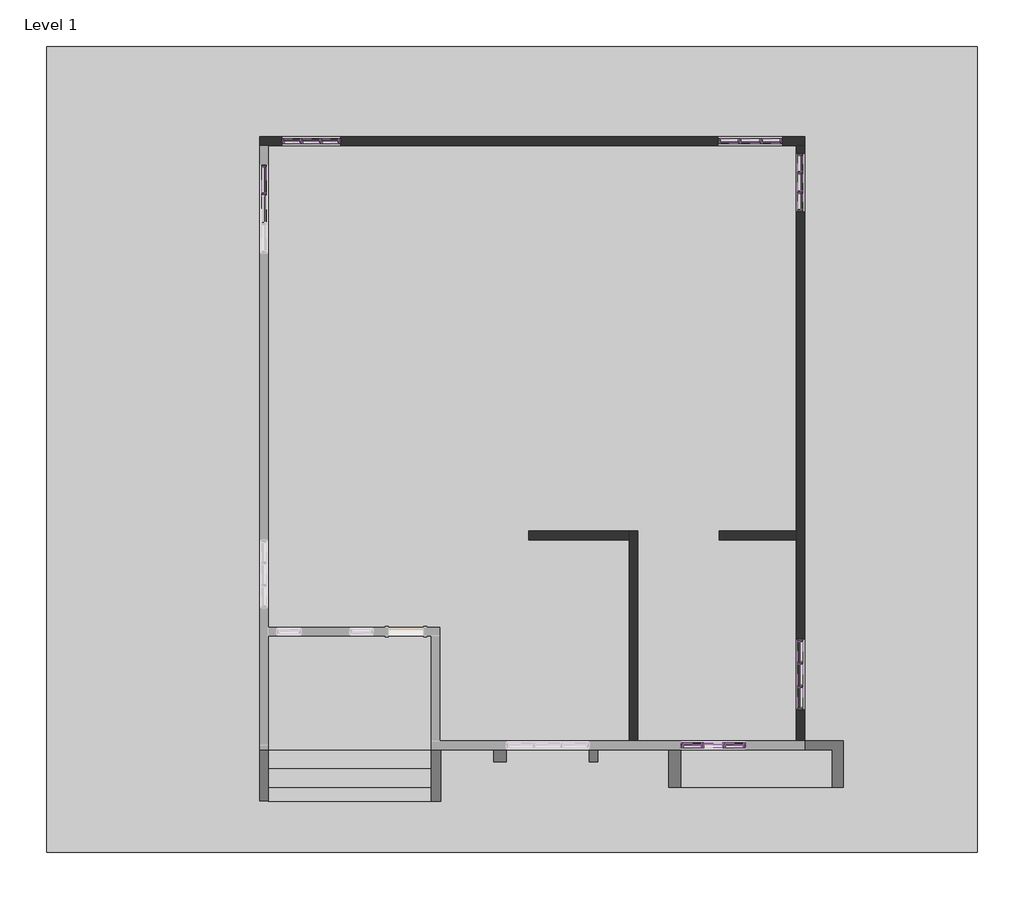
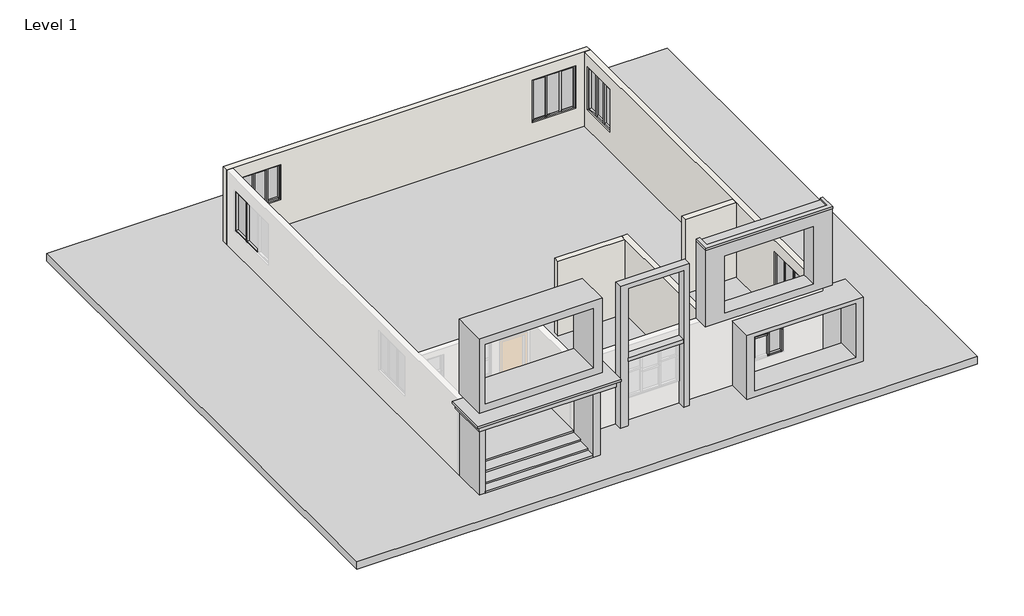
# One storey, part 2 of 2: 63 members, 17 plates, 5 walls, 3 proxies.
"""IFC4 building model written with IfcOpenShell, lengths in millimetres."""

from ifc_helpers import new_model, si_unit, origin, origin_with_axes, place, context, project, spatial, polyline, outline, extrude, faceted_brep, transform, mapped, element, save
from components import generic_models_1_generic_models_1_86db66c4, generic_models_2_generic_models_2_479a3e6c, generic_models_3_generic_models_3_c3ffb0d4, member_a980948f, member_0b7646a3, member_6494088e, member_067e20b4, member_dc106669, member_bc7dbe04, member_e7b07674, member_3cb18284, member_2ebf4a73, member_5535eeb3, member_5ecc8567, member_4301f95b, member_663484d3, member_4cf64162, member_c33c434a, member_d74592ed, member_b955a9e9, member_67d70a96, member_59fcad1a, member_8b7748c8, member_1df11e17, member_fb13da3b, member_2944fbe8, member_cfc5edb3, member_a99653d8, member_9ab3e039, system_panel_glazed_d57a6885, system_panel_glazed_a2ae5ad6, system_panel_glazed_ae4f7e76, system_panel_glazed_3d937ce6, system_panel_glazed_096f46ea, system_panel_glazed_a6fbc2a7, system_panel_glazed_9ae411f7, system_panel_glazed_f5573ca5, system_panel_glazed_7de79e50, system_panel_glazed_40386fdd, system_panel_glazed_cb1b45af, system_panel_glazed_713e3d92

model = new_model("IFC4")

# Units and contexts
model_context = context("Model", 3, world=origin())
ifc_project = project(units=[si_unit("LENGTHUNIT", "METRE", prefix="MILLI")], contexts=[model_context])

# Site, building, storey
site = spatial("IfcSite", under=ifc_project)
building = spatial("IfcBuilding", under=site)
storey = spatial("IfcBuildingStorey", under=building, Name="Level 1", Elevation=0.0)

# Proxies
placement = place(None, origin())
generic_models_1_generic_models_1_shape = generic_models_1_generic_models_1_86db66c4(model_context)
element("IfcBuildingElementProxy", 1, Name="Generic Models 1 : Generic Models 1", ObjectType="Generic Models 1 : Generic Models 1", at=placement, inside=storey, context=model_context, shape_type="MappedRepresentation", body=[
    mapped(generic_models_1_generic_models_1_shape, transform((0.0, 0.0, 0.0), x_axis=(1.0, 0.0, 0.0), y_axis=(0.0, 1.0, 0.0), z_axis=(0.0, 0.0, 1.0))),
])
generic_models_2_generic_models_2_shape = generic_models_2_generic_models_2_479a3e6c(model_context)
element("IfcBuildingElementProxy", 2, Name="Generic Models 2 : Generic Models 2", ObjectType="Generic Models 2 : Generic Models 2", at=placement, inside=storey, context=model_context, shape_type="MappedRepresentation", body=[
    mapped(generic_models_2_generic_models_2_shape, transform((0.0, 0.0, 0.0), x_axis=(1.0, 0.0, 0.0), y_axis=(0.0, 1.0, 0.0), z_axis=(0.0, 0.0, 1.0))),
])
generic_models_3_generic_models_3_shape = generic_models_3_generic_models_3_c3ffb0d4(model_context)
element("IfcBuildingElementProxy", 3, Name="Generic Models 3 : Generic Models 3", ObjectType="Generic Models 3 : Generic Models 3", at=placement, inside=storey, context=model_context, shape_type="MappedRepresentation", body=[
    mapped(generic_models_3_generic_models_3_shape, transform((0.0, 0.0, 0.0), x_axis=(1.0, 0.0, 0.0), y_axis=(0.0, 1.0, 0.0), z_axis=(0.0, 0.0, 1.0))),
])

# Members
member_shape = member_a980948f(model_context)
element("IfcMember", 4, ObjectType="Rectangular Mullion : 2.5\" x 5\" rectangular", at=placement, inside=storey, context=model_context, shape_type="MappedRepresentation", body=[
    mapped(member_shape, transform((-7907.2097681, -12030.5839922, 2596.6756637), x_axis=(0.0, 0.0, 1.0), y_axis=(1.0, 0.0, 0.0), z_axis=(0.0, 1.0, 0.0))),
])
member_2_shape = member_0b7646a3(model_context)
element("IfcMember", 5, ObjectType="Rectangular Mullion : 2.5\" x 5\" rectangular", at=placement, inside=storey, context=model_context, shape_type="MappedRepresentation", body=[
    mapped(member_2_shape, transform((-7907.2097681, -12640.1839922, 2596.6756637), x_axis=(0.0, 0.0, 1.0), y_axis=(1.0, 0.0, 0.0), z_axis=(0.0, 1.0, 0.0))),
])
element("IfcMember", 6, ObjectType="Rectangular Mullion : 2.5\" x 5\" rectangular", at=placement, inside=storey, context=model_context, shape_type="MappedRepresentation", body=[
    mapped(member_2_shape, transform((-7907.2097681, -11452.7339922, 2596.6756637), x_axis=(0.0, 0.0, 1.0), y_axis=(1.0, 0.0, 0.0), z_axis=(0.0, 1.0, 0.0))),
])
member_3_shape = member_6494088e(model_context)
element("IfcMember", 7, ObjectType="Rectangular Mullion : 2.5\" x 5\" rectangular", at=placement, inside=storey, context=model_context, shape_type="MappedRepresentation", body=[
    mapped(member_3_shape, transform((-7907.2097681, -12608.4339922, 956.4916691), x_axis=(0.0, 1.0, 0.0), y_axis=(1.0, 0.0, 0.0), z_axis=(0.0, 0.0, -1.0))),
])
element("IfcMember", 8, ObjectType="Rectangular Mullion : 2.5\" x 5\" rectangular", at=placement, inside=storey, context=model_context, shape_type="MappedRepresentation", body=[
    mapped(member_3_shape, transform((-7907.2097681, -11998.8339922, 956.4916691), x_axis=(0.0, 1.0, 0.0), y_axis=(1.0, 0.0, 0.0), z_axis=(0.0, 0.0, -1.0))),
])
element("IfcMember", 9, ObjectType="Rectangular Mullion : 2.5\" x 5\" rectangular", at=placement, inside=storey, context=model_context, shape_type="MappedRepresentation", body=[
    mapped(member_2_shape, transform((-7907.2097681, -11967.0839922, 956.4916691), x_axis=(0.0, 0.0, -1.0), y_axis=(1.0, 0.0, 0.0), z_axis=(0.0, -1.0, 0.0))),
])
element("IfcMember", 10, ObjectType="Rectangular Mullion : 2.5\" x 5\" rectangular", at=placement, inside=storey, context=model_context, shape_type="MappedRepresentation", body=[
    mapped(member_2_shape, transform((-7907.2097681, -13154.5339922, 956.4916691), x_axis=(0.0, 0.0, -1.0), y_axis=(1.0, 0.0, 0.0), z_axis=(0.0, -1.0, 0.0))),
])
element("IfcMember", 11, ObjectType="Rectangular Mullion : 2.5\" x 5\" rectangular", at=placement, inside=storey, context=model_context, shape_type="MappedRepresentation", body=[
    mapped(member_shape, transform((-7907.2097681, -12576.6839922, 956.4916691), x_axis=(0.0, 0.0, -1.0), y_axis=(1.0, 0.0, 0.0), z_axis=(0.0, -1.0, 0.0))),
])
member_4_shape = member_067e20b4(model_context)
element("IfcMember", 12, ObjectType="Rectangular Mullion : 2.5\" x 5\" rectangular", at=placement, inside=storey, context=model_context, shape_type="MappedRepresentation", body=[
    mapped(member_4_shape, transform((-7907.2097681, -11389.2339922, 956.4916691), x_axis=(0.0, 1.0, 0.0), y_axis=(1.0, 0.0, 0.0), z_axis=(0.0, 0.0, -1.0))),
])
element("IfcMember", 13, ObjectType="Rectangular Mullion : 2.5\" x 5\" rectangular", at=placement, inside=storey, context=model_context, shape_type="MappedRepresentation", body=[
    mapped(member_4_shape, transform((-7907.2097681, -13218.0339922, 2596.6756637), x_axis=(0.0, -1.0, 0.0), y_axis=(1.0, 0.0, 0.0), z_axis=(0.0, 0.0, 1.0))),
])
member_5_shape = member_dc106669(model_context)
element("IfcMember", 14, ObjectType="Rectangular Mullion : 2.5\" x 5\" rectangular", at=placement, inside=storey, context=model_context, shape_type="MappedRepresentation", body=[
    mapped(member_5_shape, transform((-7907.2097681, 669.4160078, 2556.6972088), x_axis=(0.0, 0.0, 1.0), y_axis=(-1.0, 0.0, 0.0), z_axis=(0.0, -1.0, 0.0))),
])
element("IfcMember", 15, ObjectType="Rectangular Mullion : 2.5\" x 5\" rectangular", at=placement, inside=storey, context=model_context, shape_type="MappedRepresentation", body=[
    mapped(member_5_shape, transform((-7907.2097681, -314.8339922, 2556.6972088), x_axis=(0.0, 0.0, 1.0), y_axis=(-1.0, 0.0, 0.0), z_axis=(0.0, -1.0, 0.0))),
])
element("IfcMember", 16, ObjectType="Rectangular Mullion : 2.5\" x 5\" rectangular", at=placement, inside=storey, context=model_context, shape_type="MappedRepresentation", body=[
    mapped(member_5_shape, transform((-20804.0597681, 1450.4660078, 2547.9984986), x_axis=(0.0, 0.0, 1.0), y_axis=(0.0, -1.0, 0.0), z_axis=(1.0, 0.0, 0.0))),
])
element("IfcMember", 17, ObjectType="Rectangular Mullion : 2.5\" x 5\" rectangular", at=placement, inside=storey, context=model_context, shape_type="MappedRepresentation", body=[
    mapped(member_5_shape, transform((-19819.8097681, 1450.4660078, 2547.9984986), x_axis=(0.0, 0.0, 1.0), y_axis=(0.0, -1.0, 0.0), z_axis=(1.0, 0.0, 0.0))),
])
member_6_shape = member_bc7dbe04(model_context)
element("IfcMember", 18, ObjectType="Rectangular Mullion : 2.5\" x 5\" rectangular", at=placement, inside=storey, context=model_context, shape_type="MappedRepresentation", body=[
    mapped(member_6_shape, transform((-7907.2097681, 161.4160078, 2556.6972088), x_axis=(0.0, 0.0, 1.0), y_axis=(-1.0, 0.0, 0.0), z_axis=(0.0, -1.0, 0.0))),
])
element("IfcMember", 19, ObjectType="Rectangular Mullion : 2.5\" x 5\" rectangular", at=placement, inside=storey, context=model_context, shape_type="MappedRepresentation", body=[
    mapped(member_6_shape, transform((-20296.0597681, 1450.4660078, 2547.9984986), x_axis=(0.0, 0.0, 1.0), y_axis=(0.0, -1.0, 0.0), z_axis=(1.0, 0.0, 0.0))),
])
member_7_shape = member_e7b07674(model_context)
element("IfcMember", 20, ObjectType="Rectangular Mullion : 2.5\" x 5\" rectangular", at=placement, inside=storey, context=model_context, shape_type="MappedRepresentation", body=[
    mapped(member_7_shape, transform((-7907.2097681, 129.6660078, 799.4224099), x_axis=(0.0, -1.0, 0.0), y_axis=(-1.0, 0.0, 0.0), z_axis=(0.0, 0.0, -1.0))),
])
element("IfcMember", 21, ObjectType="Rectangular Mullion : 2.5\" x 5\" rectangular", at=placement, inside=storey, context=model_context, shape_type="MappedRepresentation", body=[
    mapped(member_7_shape, transform((-7907.2097681, 637.6660078, 799.4224099), x_axis=(0.0, -1.0, 0.0), y_axis=(-1.0, 0.0, 0.0), z_axis=(0.0, 0.0, -1.0))),
])
element("IfcMember", 22, ObjectType="Rectangular Mullion : 2.5\" x 5\" rectangular", at=placement, inside=storey, context=model_context, shape_type="MappedRepresentation", body=[
    mapped(member_6_shape, transform((-7907.2097681, 605.9160078, 799.4224099), x_axis=(0.0, 0.0, -1.0), y_axis=(-1.0, 0.0, 0.0), z_axis=(0.0, 1.0, 0.0))),
])
element("IfcMember", 23, ObjectType="Rectangular Mullion : 2.5\" x 5\" rectangular", at=placement, inside=storey, context=model_context, shape_type="MappedRepresentation", body=[
    mapped(member_6_shape, transform((-20740.5597681, 1450.4660078, 1117.1565965), x_axis=(0.0, 0.0, -1.0), y_axis=(0.0, -1.0, 0.0), z_axis=(-1.0, 0.0, 0.0))),
])
element("IfcMember", 24, ObjectType="Rectangular Mullion : 2.5\" x 5\" rectangular", at=placement, inside=storey, context=model_context, shape_type="MappedRepresentation", body=[
    mapped(member_5_shape, transform((-7907.2097681, 97.9160078, 799.4224099), x_axis=(0.0, 0.0, -1.0), y_axis=(-1.0, 0.0, 0.0), z_axis=(0.0, 1.0, 0.0))),
])
element("IfcMember", 25, ObjectType="Rectangular Mullion : 2.5\" x 5\" rectangular", at=placement, inside=storey, context=model_context, shape_type="MappedRepresentation", body=[
    mapped(member_5_shape, transform((-7907.2097681, 1082.1660078, 799.4224099), x_axis=(0.0, 0.0, -1.0), y_axis=(-1.0, 0.0, 0.0), z_axis=(0.0, 1.0, 0.0))),
])
element("IfcMember", 26, ObjectType="Rectangular Mullion : 2.5\" x 5\" rectangular", at=placement, inside=storey, context=model_context, shape_type="MappedRepresentation", body=[
    mapped(member_5_shape, transform((-20232.5597681, 1450.4660078, 1117.1565965), x_axis=(0.0, 0.0, -1.0), y_axis=(0.0, -1.0, 0.0), z_axis=(-1.0, 0.0, 0.0))),
])
element("IfcMember", 27, ObjectType="Rectangular Mullion : 2.5\" x 5\" rectangular", at=placement, inside=storey, context=model_context, shape_type="MappedRepresentation", body=[
    mapped(member_5_shape, transform((-21216.8097681, 1450.4660078, 1117.1565965), x_axis=(0.0, 0.0, -1.0), y_axis=(0.0, -1.0, 0.0), z_axis=(-1.0, 0.0, 0.0))),
])
member_8_shape = member_3cb18284(model_context)
element("IfcMember", 28, ObjectType="Rectangular Mullion : 2.5\" x 5\" rectangular", at=placement, inside=storey, context=model_context, shape_type="MappedRepresentation", body=[
    mapped(member_8_shape, transform((-7907.2097681, 1145.6660078, 2556.6972088), x_axis=(0.0, 1.0, 0.0), y_axis=(-1.0, 0.0, 0.0), z_axis=(0.0, 0.0, 1.0))),
])
element("IfcMember", 29, ObjectType="Rectangular Mullion : 2.5\" x 5\" rectangular", at=placement, inside=storey, context=model_context, shape_type="MappedRepresentation", body=[
    mapped(member_8_shape, transform((-7907.2097681, -378.3339922, 799.4224099), x_axis=(0.0, -1.0, 0.0), y_axis=(-1.0, 0.0, 0.0), z_axis=(0.0, 0.0, -1.0))),
])
member_9_shape = member_2ebf4a73(model_context)
element("IfcMember", 30, ObjectType="Rectangular Mullion : 2.5\" x 5\" rectangular", at=placement, inside=storey, context=model_context, shape_type="MappedRepresentation", body=[
    mapped(member_9_shape, transform((-9450.2597681, 1450.4660078, 2596.0086756), x_axis=(0.0, 0.0, 1.0), y_axis=(0.0, 1.0, 0.0), z_axis=(-1.0, 0.0, 0.0))),
])
element("IfcMember", 31, ObjectType="Rectangular Mullion : 2.5\" x 5\" rectangular", at=placement, inside=storey, context=model_context, shape_type="MappedRepresentation", body=[
    mapped(member_9_shape, transform((-9907.4597681, -14132.4339922, 2463.7993261), x_axis=(0.0, 0.0, 1.0), y_axis=(0.0, -1.0, 0.0), z_axis=(1.0, 0.0, 0.0))),
])
member_10_shape = member_5535eeb3(model_context)
element("IfcMember", 32, ObjectType="Rectangular Mullion : 2.5\" x 5\" rectangular", at=placement, inside=storey, context=model_context, shape_type="MappedRepresentation", body=[
    mapped(member_10_shape, transform((-8891.4597681, 1450.4660078, 2596.0086756), x_axis=(0.0, 0.0, 1.0), y_axis=(0.0, 1.0, 0.0), z_axis=(-1.0, 0.0, 0.0))),
])
element("IfcMember", 33, ObjectType="Rectangular Mullion : 2.5\" x 5\" rectangular", at=placement, inside=storey, context=model_context, shape_type="MappedRepresentation", body=[
    mapped(member_10_shape, transform((-9977.3097681, 1450.4660078, 2596.0086756), x_axis=(0.0, 0.0, 1.0), y_axis=(0.0, 1.0, 0.0), z_axis=(-1.0, 0.0, 0.0))),
])
element("IfcMember", 34, ObjectType="Rectangular Mullion : 2.5\" x 5\" rectangular", at=placement, inside=storey, context=model_context, shape_type="MappedRepresentation", body=[
    mapped(member_10_shape, transform((-9380.4097681, -14132.4339922, 2463.7993261), x_axis=(0.0, 0.0, 1.0), y_axis=(0.0, -1.0, 0.0), z_axis=(1.0, 0.0, 0.0))),
])
member_11_shape = member_5ecc8567(model_context)
element("IfcMember", 35, ObjectType="Rectangular Mullion : 2.5\" x 5\" rectangular", at=placement, inside=storey, context=model_context, shape_type="MappedRepresentation", body=[
    mapped(member_11_shape, transform((-8923.2097681, 1450.4660078, 867.8712232), x_axis=(-1.0, 0.0, 0.0), y_axis=(0.0, 1.0, 0.0), z_axis=(0.0, 0.0, -1.0))),
])
element("IfcMember", 36, ObjectType="Rectangular Mullion : 2.5\" x 5\" rectangular", at=placement, inside=storey, context=model_context, shape_type="MappedRepresentation", body=[
    mapped(member_11_shape, transform((-9482.0097681, 1450.4660078, 867.8712232), x_axis=(-1.0, 0.0, 0.0), y_axis=(0.0, 1.0, 0.0), z_axis=(0.0, 0.0, -1.0))),
])
element("IfcMember", 37, ObjectType="Rectangular Mullion : 2.5\" x 5\" rectangular", at=placement, inside=storey, context=model_context, shape_type="MappedRepresentation", body=[
    mapped(member_10_shape, transform((-9513.7597681, 1450.4660078, 867.8712232), x_axis=(0.0, 0.0, -1.0), y_axis=(0.0, 1.0, 0.0), z_axis=(1.0, 0.0, 0.0))),
])
element("IfcMember", 38, ObjectType="Rectangular Mullion : 2.5\" x 5\" rectangular", at=placement, inside=storey, context=model_context, shape_type="MappedRepresentation", body=[
    mapped(member_10_shape, transform((-8427.9097681, 1450.4660078, 867.8712232), x_axis=(0.0, 0.0, -1.0), y_axis=(0.0, 1.0, 0.0), z_axis=(1.0, 0.0, 0.0))),
])
element("IfcMember", 39, ObjectType="Rectangular Mullion : 2.5\" x 5\" rectangular", at=placement, inside=storey, context=model_context, shape_type="MappedRepresentation", body=[
    mapped(member_10_shape, transform((-9843.9597681, -14132.4339922, 684.1737808), x_axis=(0.0, 0.0, -1.0), y_axis=(0.0, -1.0, 0.0), z_axis=(-1.0, 0.0, 0.0))),
])
element("IfcMember", 40, ObjectType="Rectangular Mullion : 2.5\" x 5\" rectangular", at=placement, inside=storey, context=model_context, shape_type="MappedRepresentation", body=[
    mapped(member_10_shape, transform((-10929.8097681, -14132.4339922, 684.1737808), x_axis=(0.0, 0.0, -1.0), y_axis=(0.0, -1.0, 0.0), z_axis=(-1.0, 0.0, 0.0))),
])
element("IfcMember", 41, ObjectType="Rectangular Mullion : 2.5\" x 5\" rectangular", at=placement, inside=storey, context=model_context, shape_type="MappedRepresentation", body=[
    mapped(member_9_shape, transform((-8954.9597681, 1450.4660078, 867.8712232), x_axis=(0.0, 0.0, -1.0), y_axis=(0.0, 1.0, 0.0), z_axis=(1.0, 0.0, 0.0))),
])
member_12_shape = member_4301f95b(model_context)
element("IfcMember", 42, ObjectType="Rectangular Mullion : 2.5\" x 5\" rectangular", at=placement, inside=storey, context=model_context, shape_type="MappedRepresentation", body=[
    mapped(member_12_shape, transform((-10040.8097681, 1450.4660078, 867.8712232), x_axis=(-1.0, 0.0, 0.0), y_axis=(0.0, 1.0, 0.0), z_axis=(0.0, 0.0, -1.0))),
])
element("IfcMember", 43, ObjectType="Rectangular Mullion : 2.5\" x 5\" rectangular", at=placement, inside=storey, context=model_context, shape_type="MappedRepresentation", body=[
    mapped(member_12_shape, transform((-8364.4097681, 1450.4660078, 2596.0086756), x_axis=(1.0, 0.0, 0.0), y_axis=(0.0, 1.0, 0.0), z_axis=(0.0, 0.0, 1.0))),
])
member_13_shape = member_663484d3(model_context)
element("IfcMember", 44, ObjectType="Rectangular Mullion : 2.5\" x 5\" rectangular", at=placement, inside=storey, context=model_context, shape_type="MappedRepresentation", body=[
    mapped(member_13_shape, transform((-20264.3097681, 1450.4660078, 1117.1565965), x_axis=(1.0, 0.0, 0.0), y_axis=(0.0, -1.0, 0.0), z_axis=(0.0, 0.0, -1.0))),
])
element("IfcMember", 45, ObjectType="Rectangular Mullion : 2.5\" x 5\" rectangular", at=placement, inside=storey, context=model_context, shape_type="MappedRepresentation", body=[
    mapped(member_13_shape, transform((-20772.3097681, 1450.4660078, 1117.1565965), x_axis=(1.0, 0.0, 0.0), y_axis=(0.0, -1.0, 0.0), z_axis=(0.0, 0.0, -1.0))),
])
member_14_shape = member_4cf64162(model_context)
element("IfcMember", 46, ObjectType="Rectangular Mullion : 2.5\" x 5\" rectangular", at=placement, inside=storey, context=model_context, shape_type="MappedRepresentation", body=[
    mapped(member_14_shape, transform((-21280.3097681, 1450.4660078, 2547.9984986), x_axis=(-1.0, 0.0, 0.0), y_axis=(0.0, -1.0, 0.0), z_axis=(0.0, 0.0, 1.0))),
])
element("IfcMember", 47, ObjectType="Rectangular Mullion : 2.5\" x 5\" rectangular", at=placement, inside=storey, context=model_context, shape_type="MappedRepresentation", body=[
    mapped(member_14_shape, transform((-19756.3097681, 1450.4660078, 1117.1565965), x_axis=(1.0, 0.0, 0.0), y_axis=(0.0, -1.0, 0.0), z_axis=(0.0, 0.0, -1.0))),
])
member_15_shape = member_c33c434a(model_context)
element("IfcMember", 48, ObjectType="Rectangular Mullion : 2.5\" x 5\" rectangular", at=placement, inside=storey, context=model_context, shape_type="MappedRepresentation", body=[
    mapped(member_15_shape, transform((-21737.5097681, 110.6160078, 2530.4981779), x_axis=(0.0, 0.0, 1.0), y_axis=(-1.0, 0.0, 0.0), z_axis=(0.0, -1.0, 0.0))),
])
member_16_shape = member_d74592ed(model_context)
element("IfcMember", 49, ObjectType="Rectangular Mullion : 2.5\" x 5\" rectangular", at=placement, inside=storey, context=model_context, shape_type="MappedRepresentation", body=[
    mapped(member_16_shape, transform((-21737.5097681, 78.8660078, 850.000156), x_axis=(0.0, -1.0, 0.0), y_axis=(-1.0, 0.0, 0.0), z_axis=(0.0, 0.0, -1.0))),
])
element("IfcMember", 50, ObjectType="Rectangular Mullion : 2.5\" x 5\" rectangular", at=placement, inside=storey, context=model_context, shape_type="MappedRepresentation", body=[
    mapped(member_15_shape, transform((-21737.5097681, 777.3660078, 850.000156), x_axis=(0.0, 0.0, -1.0), y_axis=(-1.0, 0.0, 0.0), z_axis=(0.0, 1.0, 0.0))),
])
member_17_shape = member_b955a9e9(model_context)
element("IfcMember", 51, ObjectType="Rectangular Mullion : 2.5\" x 5\" rectangular", at=placement, inside=storey, context=model_context, shape_type="MappedRepresentation", body=[
    mapped(member_17_shape, transform((-21737.5097681, 47.1160078, 850.000156), x_axis=(0.0, 0.0, -1.0), y_axis=(-1.0, 0.0, 0.0), z_axis=(0.0, 1.0, 0.0))),
])
member_18_shape = member_67d70a96(model_context)
element("IfcMember", 52, ObjectType="Rectangular Mullion : 2.5\" x 5\" rectangular", at=placement, inside=storey, context=model_context, shape_type="MappedRepresentation", body=[
    mapped(member_18_shape, transform((-21737.5097681, 840.8660078, 2530.4981779), x_axis=(0.0, 1.0, 0.0), y_axis=(-1.0, 0.0, 0.0), z_axis=(0.0, 0.0, 1.0))),
])
member_19_shape = member_59fcad1a(model_context)
element("IfcMember", 53, ObjectType="Rectangular Mullion : 2.5\" x 5\" rectangular", at=placement, inside=storey, context=model_context, shape_type="MappedRepresentation", body=[
    mapped(member_19_shape, transform((-9316.9097681, -14132.4339922, 684.1737808), x_axis=(1.0, 0.0, 0.0), y_axis=(0.0, -1.0, 0.0), z_axis=(0.0, 0.0, -1.0))),
])
element("IfcMember", 54, ObjectType="Rectangular Mullion : 2.5\" x 5\" rectangular", at=placement, inside=storey, context=model_context, shape_type="MappedRepresentation", body=[
    mapped(member_19_shape, transform((-10993.3097681, -14132.4339922, 1573.9865534), x_axis=(-1.0, 0.0, 0.0), y_axis=(0.0, -1.0, 0.0), z_axis=(0.0, 0.0, 1.0))),
])
member_20_shape = member_8b7748c8(model_context)
element("IfcMember", 55, ObjectType="Rectangular Mullion : 2.5\" x 5\" rectangular", at=placement, inside=storey, context=model_context, shape_type="MappedRepresentation", body=[
    mapped(member_20_shape, transform((-10434.5097681, -14132.4339922, 1675.5865534), x_axis=(1.0, 0.0, 0.0), y_axis=(0.0, -1.0, 0.0), z_axis=(0.0, 0.0, -1.0))),
])
element("IfcMember", 56, ObjectType="Rectangular Mullion : 2.5\" x 5\" rectangular", at=placement, inside=storey, context=model_context, shape_type="MappedRepresentation", body=[
    mapped(member_20_shape, transform((-9875.7097681, -14132.4339922, 1675.5865534), x_axis=(1.0, 0.0, 0.0), y_axis=(0.0, -1.0, 0.0), z_axis=(0.0, 0.0, -1.0))),
])
member_21_shape = member_1df11e17(model_context)
element("IfcMember", 57, ObjectType="Rectangular Mullion : 2.5\" x 5\" rectangular", at=placement, inside=storey, context=model_context, shape_type="MappedRepresentation", body=[
    mapped(member_21_shape, transform((-9380.4097681, -14132.4339922, 1675.5865534), x_axis=(0.0, 0.0, 1.0), y_axis=(0.0, -1.0, 0.0), z_axis=(1.0, 0.0, 0.0))),
])
element("IfcMember", 58, ObjectType="Rectangular Mullion : 2.5\" x 5\" rectangular", at=placement, inside=storey, context=model_context, shape_type="MappedRepresentation", body=[
    mapped(member_21_shape, transform((-10466.2597681, -14132.4339922, 1675.5865534), x_axis=(0.0, 0.0, 1.0), y_axis=(0.0, -1.0, 0.0), z_axis=(1.0, 0.0, 0.0))),
])
member_22_shape = member_fb13da3b(model_context)
element("IfcMember", 59, ObjectType="Rectangular Mullion : 2.5\" x 5\" rectangular", at=placement, inside=storey, context=model_context, shape_type="MappedRepresentation", body=[
    mapped(member_22_shape, transform((-9316.9097681, -14132.4339922, 1573.9865534), x_axis=(1.0, 0.0, 0.0), y_axis=(0.0, -1.0, 0.0), z_axis=(0.0, 0.0, -1.0))),
])
element("IfcMember", 60, ObjectType="Rectangular Mullion : 2.5\" x 5\" rectangular", at=placement, inside=storey, context=model_context, shape_type="MappedRepresentation", body=[
    mapped(member_22_shape, transform((-10993.3097681, -14132.4339922, 1675.5865534), x_axis=(-1.0, 0.0, 0.0), y_axis=(0.0, -1.0, 0.0), z_axis=(0.0, 0.0, 1.0))),
])
member_23_shape = member_2944fbe8(model_context)
element("IfcMember", 61, ObjectType="Rectangular Mullion : 2.5\" x 5\" rectangular", at=placement, inside=storey, context=model_context, shape_type="MappedRepresentation", body=[
    mapped(member_23_shape, transform((-9316.9097681, -14132.4339922, 1675.5865534), x_axis=(1.0, 0.0, 0.0), y_axis=(0.0, -1.0, 0.0), z_axis=(0.0, 0.0, -1.0))),
])
member_24_shape = member_cfc5edb3(model_context)
element("IfcMember", 62, ObjectType="Rectangular Mullion : 2.5\" x 5\" rectangular", at=placement, inside=storey, context=model_context, shape_type="MappedRepresentation", body=[
    mapped(member_24_shape, transform((-10434.5097681, -14132.4339922, 1573.9865534), x_axis=(1.0, 0.0, 0.0), y_axis=(0.0, -1.0, 0.0), z_axis=(0.0, 0.0, -1.0))),
])
element("IfcMember", 63, ObjectType="Rectangular Mullion : 2.5\" x 5\" rectangular", at=placement, inside=storey, context=model_context, shape_type="MappedRepresentation", body=[
    mapped(member_24_shape, transform((-9875.7097681, -14132.4339922, 1573.9865534), x_axis=(1.0, 0.0, 0.0), y_axis=(0.0, -1.0, 0.0), z_axis=(0.0, 0.0, -1.0))),
])
member_25_shape = member_a99653d8(model_context)
element("IfcMember", 64, ObjectType="Rectangular Mullion : 2.5\" x 5\" rectangular", at=placement, inside=storey, context=model_context, shape_type="MappedRepresentation", body=[
    mapped(member_25_shape, transform((-10434.5097681, -14132.4339922, 684.1737808), x_axis=(1.0, 0.0, 0.0), y_axis=(0.0, -1.0, 0.0), z_axis=(0.0, 0.0, -1.0))),
])
element("IfcMember", 65, ObjectType="Rectangular Mullion : 2.5\" x 5\" rectangular", at=placement, inside=storey, context=model_context, shape_type="MappedRepresentation", body=[
    mapped(member_25_shape, transform((-9875.7097681, -14132.4339922, 684.1737808), x_axis=(1.0, 0.0, 0.0), y_axis=(0.0, -1.0, 0.0), z_axis=(0.0, 0.0, -1.0))),
])
member_26_shape = member_9ab3e039(model_context)
element("IfcMember", 66, ObjectType="Rectangular Mullion : 2.5\" x 5\" rectangular", at=placement, inside=storey, context=model_context, shape_type="MappedRepresentation", body=[
    mapped(member_26_shape, transform((-9907.4597681, -14132.4339922, 1573.9865534), x_axis=(0.0, 0.0, 1.0), y_axis=(0.0, -1.0, 0.0), z_axis=(1.0, 0.0, 0.0))),
])

# Plates
system_panel_glazed_shape = system_panel_glazed_d57a6885(model_context)
element("IfcPlate", 67, ObjectType="System Panel : Glazed", at=placement, inside=storey, context=model_context, shape_type="MappedRepresentation", body=[
    mapped(system_panel_glazed_shape, transform((-7907.2097681, -12897.3589922, 1019.9916691), x_axis=(0.0, 1.0, 0.0), y_axis=(-1.0, 0.0, 0.0), z_axis=(0.0, 0.0, 1.0))),
])
element("IfcPlate", 68, ObjectType="System Panel : Glazed", at=placement, inside=storey, context=model_context, shape_type="MappedRepresentation", body=[
    mapped(system_panel_glazed_shape, transform((-7907.2097681, -11709.9089922, 1019.9916691), x_axis=(0.0, 1.0, 0.0), y_axis=(-1.0, 0.0, 0.0), z_axis=(0.0, 0.0, 1.0))),
])
system_panel_glazed_2_shape = system_panel_glazed_a2ae5ad6(model_context)
element("IfcPlate", 69, ObjectType="System Panel : Glazed", at=placement, inside=storey, context=model_context, shape_type="MappedRepresentation", body=[
    mapped(system_panel_glazed_2_shape, transform((-7907.2097681, -12303.6339922, 1019.9916691), x_axis=(0.0, 1.0, 0.0), y_axis=(-1.0, 0.0, 0.0), z_axis=(0.0, 0.0, 1.0))),
])
system_panel_glazed_3_shape = system_panel_glazed_ae4f7e76(model_context)
element("IfcPlate", 70, ObjectType="System Panel : Glazed", at=placement, inside=storey, context=model_context, shape_type="MappedRepresentation", body=[
    mapped(system_panel_glazed_3_shape, transform((-7907.2097681, 875.7910078, 862.9224099), x_axis=(0.0, -1.0, 0.0), y_axis=(1.0, 0.0, 0.0), z_axis=(0.0, 0.0, 1.0))),
])
element("IfcPlate", 71, ObjectType="System Panel : Glazed", at=placement, inside=storey, context=model_context, shape_type="MappedRepresentation", body=[
    mapped(system_panel_glazed_3_shape, transform((-7907.2097681, -108.4589922, 862.9224099), x_axis=(0.0, -1.0, 0.0), y_axis=(1.0, 0.0, 0.0), z_axis=(0.0, 0.0, 1.0))),
])
system_panel_glazed_4_shape = system_panel_glazed_3d937ce6(model_context)
element("IfcPlate", 72, ObjectType="System Panel : Glazed", at=placement, inside=storey, context=model_context, shape_type="MappedRepresentation", body=[
    mapped(system_panel_glazed_4_shape, transform((-7907.2097681, 383.6660078, 862.9224099), x_axis=(0.0, -1.0, 0.0), y_axis=(1.0, 0.0, 0.0), z_axis=(0.0, 0.0, 1.0))),
])
system_panel_glazed_5_shape = system_panel_glazed_096f46ea(model_context)
element("IfcPlate", 73, ObjectType="System Panel : Glazed", at=placement, inside=storey, context=model_context, shape_type="MappedRepresentation", body=[
    mapped(system_panel_glazed_5_shape, transform((-8659.6847681, 1450.4660078, 931.3712232), x_axis=(-1.0, 0.0, 0.0), y_axis=(0.0, -1.0, 0.0), z_axis=(0.0, 0.0, 1.0))),
])
element("IfcPlate", 74, ObjectType="System Panel : Glazed", at=placement, inside=storey, context=model_context, shape_type="MappedRepresentation", body=[
    mapped(system_panel_glazed_5_shape, transform((-9745.5347681, 1450.4660078, 931.3712232), x_axis=(-1.0, 0.0, 0.0), y_axis=(0.0, -1.0, 0.0), z_axis=(0.0, 0.0, 1.0))),
])
system_panel_glazed_6_shape = system_panel_glazed_a6fbc2a7(model_context)
element("IfcPlate", 75, ObjectType="System Panel : Glazed", at=placement, inside=storey, context=model_context, shape_type="MappedRepresentation", body=[
    mapped(system_panel_glazed_6_shape, transform((-9202.6097681, 1450.4660078, 931.3712232), x_axis=(-1.0, 0.0, 0.0), y_axis=(0.0, -1.0, 0.0), z_axis=(0.0, 0.0, 1.0))),
])
system_panel_glazed_7_shape = system_panel_glazed_9ae411f7(model_context)
element("IfcPlate", 76, ObjectType="System Panel : Glazed", at=placement, inside=storey, context=model_context, shape_type="MappedRepresentation", body=[
    mapped(system_panel_glazed_7_shape, transform((-21010.4347681, 1450.4660078, 1180.6565965), x_axis=(1.0, 0.0, 0.0), y_axis=(0.0, 1.0, 0.0), z_axis=(0.0, 0.0, 1.0))),
])
element("IfcPlate", 77, ObjectType="System Panel : Glazed", at=placement, inside=storey, context=model_context, shape_type="MappedRepresentation", body=[
    mapped(system_panel_glazed_7_shape, transform((-20026.1847681, 1450.4660078, 1180.6565965), x_axis=(1.0, 0.0, 0.0), y_axis=(0.0, 1.0, 0.0), z_axis=(0.0, 0.0, 1.0))),
])
system_panel_glazed_8_shape = system_panel_glazed_f5573ca5(model_context)
element("IfcPlate", 78, ObjectType="System Panel : Glazed", at=placement, inside=storey, context=model_context, shape_type="MappedRepresentation", body=[
    mapped(system_panel_glazed_8_shape, transform((-20518.3097681, 1450.4660078, 1180.6565965), x_axis=(1.0, 0.0, 0.0), y_axis=(0.0, 1.0, 0.0), z_axis=(0.0, 0.0, 1.0))),
])
system_panel_glazed_9_shape = system_panel_glazed_7de79e50(model_context)
element("IfcPlate", 79, ObjectType="System Panel : Glazed", at=placement, inside=storey, context=model_context, shape_type="MappedRepresentation", body=[
    mapped(system_panel_glazed_9_shape, transform((-21737.5097681, 443.9910078, 913.500156), x_axis=(0.0, -1.0, 0.0), y_axis=(1.0, 0.0, 0.0), z_axis=(0.0, 0.0, 1.0))),
])
system_panel_glazed_10_shape = system_panel_glazed_40386fdd(model_context)
element("IfcPlate", 80, ObjectType="System Panel : Glazed", at=placement, inside=storey, context=model_context, shape_type="MappedRepresentation", body=[
    mapped(system_panel_glazed_10_shape, transform((-9612.1847681, -14132.4339922, 747.6737808), x_axis=(1.0, 0.0, 0.0), y_axis=(0.0, 1.0, 0.0), z_axis=(0.0, 0.0, 1.0))),
])
system_panel_glazed_11_shape = system_panel_glazed_cb1b45af(model_context)
element("IfcPlate", 81, ObjectType="System Panel : Glazed", at=placement, inside=storey, context=model_context, shape_type="MappedRepresentation", body=[
    mapped(system_panel_glazed_11_shape, transform((-10698.0347681, -14132.4339922, 1707.3365534), x_axis=(1.0, 0.0, 0.0), y_axis=(0.0, 1.0, 0.0), z_axis=(0.0, 0.0, 1.0))),
])
element("IfcPlate", 82, ObjectType="System Panel : Glazed", at=placement, inside=storey, context=model_context, shape_type="MappedRepresentation", body=[
    mapped(system_panel_glazed_11_shape, transform((-9612.1847681, -14132.4339922, 1707.3365534), x_axis=(1.0, 0.0, 0.0), y_axis=(0.0, 1.0, 0.0), z_axis=(0.0, 0.0, 1.0))),
])
system_panel_glazed_12_shape = system_panel_glazed_713e3d92(model_context)
element("IfcPlate", 83, ObjectType="System Panel : Glazed", at=placement, inside=storey, context=model_context, shape_type="MappedRepresentation", body=[
    mapped(system_panel_glazed_12_shape, transform((-10155.1097681, -14132.4339922, 1605.7365534), x_axis=(1.0, 0.0, 0.0), y_axis=(0.0, 1.0, 0.0), z_axis=(0.0, 0.0, 1.0))),
])

# Walls
element("IfcWall", 84, ObjectType="9\"", at=placement, inside=storey, context=model_context, shape_type="Brep", body=[
    faceted_brep([(-7792.9097681, 1564.7660078, 0.0), (-21851.8097681, 1564.7660078, 0.0), (-21851.8097681, 1564.7660078, 3048.0), (-7792.9097681, 1564.7660078, 3048.0), (-8364.4097681, 1564.7660078, 867.8712232), (-8364.4097681, 1564.7660078, 2596.0086756), (-10040.8097681, 1564.7660078, 2596.0086756), (-10040.8097681, 1564.7660078, 867.8712232), (-21280.3097681, 1564.7660078, 2547.9984986), (-21280.3097681, 1564.7660078, 1117.1565965), (-19756.3097681, 1564.7660078, 1117.1565965), (-19756.3097681, 1564.7660078, 2547.9984986), (-21851.8097681, 1336.1660078, 0.0), (-21623.2097681, 1336.1660078, 0.0), (-8021.5097681, 1336.1660078, 0.0), (-7792.9097681, 1336.1660078, 0.0), (-7792.9097681, 1336.1660078, 3048.0), (-8021.5097681, 1336.1660078, 3048.0), (-21623.2097681, 1336.1660078, 3048.0), (-21851.8097681, 1336.1660078, 3048.0), (-8364.4097681, 1336.1660078, 2596.0086756), (-8364.4097681, 1336.1660078, 867.8712232), (-10040.8097681, 1336.1660078, 867.8712232), (-10040.8097681, 1336.1660078, 2596.0086756), (-21280.3097681, 1336.1660078, 1117.1565965), (-21280.3097681, 1336.1660078, 2547.9984986), (-19756.3097681, 1336.1660078, 2547.9984986), (-19756.3097681, 1336.1660078, 1117.1565965)], [[[0, 1, 2, 3], [4, 5, 6, 7], [8, 9, 10, 11]], [[12, 13, 14, 15, 16, 17, 18, 19], [20, 21, 22, 23], [24, 25, 26, 27]], [[1, 0, 15, 14, 13, 12]], [[3, 2, 19, 18, 17, 16]], [[2, 1, 12, 19]], [[0, 3, 16, 15]], [[20, 5, 4, 21]], [[5, 20, 23, 6]], [[6, 23, 22, 7]], [[21, 4, 7, 22]], [[24, 9, 8, 25]], [[25, 8, 11, 26]], [[26, 11, 10, 27]], [[9, 24, 27, 10]]]),
])
element("IfcWall", 85, ObjectType="9\"", at=placement, inside=storey, context=model_context, shape_type="Brep", body=[
    faceted_brep([(-7792.9097681, -14018.1339922, 0.0), (-7792.9097681, 1336.1660078, 0.0), (-7792.9097681, 1336.1660078, 3048.0), (-7792.9097681, -14018.1339922, 3048.0), (-7792.9097681, -13218.0339922, 956.4916691), (-7792.9097681, -13218.0339922, 2596.6756637), (-7792.9097681, -11389.2339922, 2596.6756637), (-7792.9097681, -11389.2339922, 956.4916691), (-7792.9097681, 1145.6660078, 2556.6972088), (-7792.9097681, 1145.6660078, 799.4224099), (-7792.9097681, -378.3339922, 799.4224099), (-7792.9097681, -378.3339922, 2556.6972088), (-8021.5097681, 1336.1660078, 0.0), (-8021.5097681, -8607.9339922, 0.0), (-8021.5097681, -8836.5339922, 0.0), (-8021.5097681, -14018.1339922, 0.0), (-8021.5097681, -14018.1339922, 3048.0), (-8021.5097681, -8836.5339922, 3048.0), (-8021.5097681, -8607.9339922, 3048.0), (-8021.5097681, 1336.1660078, 3048.0), (-8021.5097681, -13218.0339922, 2596.6756637), (-8021.5097681, -13218.0339922, 956.4916691), (-8021.5097681, -11389.2339922, 956.4916691), (-8021.5097681, -11389.2339922, 2596.6756637), (-8021.5097681, 1145.6660078, 799.4224099), (-8021.5097681, 1145.6660078, 2556.6972088), (-8021.5097681, -378.3339922, 2556.6972088), (-8021.5097681, -378.3339922, 799.4224099)], [[[0, 1, 2, 3], [4, 5, 6, 7], [8, 9, 10, 11]], [[12, 13, 14, 15, 16, 17, 18, 19], [20, 21, 22, 23], [24, 25, 26, 27]], [[1, 0, 15, 14, 13, 12]], [[3, 2, 19, 18, 17, 16]], [[2, 1, 12, 19]], [[0, 3, 16, 15]], [[4, 21, 20, 5]], [[5, 20, 23, 6]], [[6, 23, 22, 7]], [[21, 4, 7, 22]], [[24, 9, 8, 25]], [[25, 8, 11, 26]], [[10, 27, 26, 11]], [[9, 24, 27, 10]]]),
])
element("IfcWall", 86, ObjectType="9\"", at=placement, inside=storey, context=model_context, shape_type="Brep", body=[
    faceted_brep([(-12098.2097681, -14018.1339922, 0.0), (-12098.2097681, -8607.9339922, 0.0), (-12098.2097681, -8607.9339922, 3048.0), (-12098.2097681, -14018.1339922, 3048.0), (-12326.8097681, -14018.1339922, 0.0), (-12326.8097681, -14018.1339922, 3048.0), (-12326.8097681, -8836.5339922, 3048.0), (-12326.8097681, -8607.9339922, 3048.0), (-12326.8097681, -8607.9339922, 0.0), (-12326.8097681, -8836.5339922, 0.0)], [[[0, 1, 2, 3]], [[4, 5, 6, 7, 8, 9]], [[1, 0, 4, 9, 8]], [[3, 2, 7, 6, 5]], [[0, 3, 5, 4]], [[2, 1, 8, 7]]]),
])
element("IfcWall", 87, ObjectType="9\"", at=placement, inside=storey, context=model_context, shape_type="SweptSolid", body=[
    extrude(outline(polyline([(-14917.6097681, -8607.9339922), (-12326.8097681, -8607.9339922), (-12326.8097681, -8836.5339922), (-14917.6097681, -8836.5339922), (-14917.6097681, -8607.9339922)])), origin_with_axes(), (0.0, 0.0, 1.0), 3048.0),
])
element("IfcWall", 88, ObjectType="9\"", at=placement, inside=storey, context=model_context, shape_type="SweptSolid", body=[
    extrude(outline(polyline([(-10002.7097681, -8607.9339922), (-8021.5097681, -8607.9339922), (-8021.5097681, -8836.5339922), (-10002.7097681, -8836.5339922), (-10002.7097681, -8607.9339922)])), origin_with_axes(), (0.0, 0.0, 1.0), 3048.0),
])

save(model, "model.ifc")

# Revit data of these elements
# Type "Rectangular Mullion : 2.5\" x 5\" rectangular"
#   built-in parameter 1007304 = 0.416667 (stored number, unit not read)
#   built-in parameter 1007301 = 0.104167 (stored number, unit not read)
#   built-in parameter 1007300 = 0.104167 (stored number, unit not read)
# Type "System Panel : Glazed"
#   Construction Type Id = "GSP4R"
#   Analytic Construction = "1/8 in Pilkington single glazing"
#   Visual Light Transmittance = 0.9
#   Solar Heat Gain Coefficient = 0.86
#   Heat Transfer Coefficient (U) = 1.18115 BTU/(h·ft²·°F)
#   Define Thermal Properties by = 1
# Type "9\""
#   Assembly Code = "B2010"
#   Layers, outside or top first: 0' - 9" no material (function 1)
# Element 1 (IfcBuildingElementProxy, "Generic Models 1 : Generic Models 1")
#   Phase Created = New Construction
# Element 2 (IfcBuildingElementProxy, "Generic Models 2 : Generic Models 2")
#   Phase Created = New Construction
# Element 3 (IfcBuildingElementProxy, "Generic Models 3 : Generic Models 3")
#   Phase Created = New Construction
# Elements 4, 5, 6, 7, 8, 9, 10, 11, 12, 13, 14, 15, 16, 17, 18, 19, 20, 21, 22, 23, 24, 25, 26, 27, 28, 29, 30, 31, 32, 33, 34, 35, 36, 37, 38, 39, 40, 41, 42, 43, 44, 45, 46, 47, 48, 49, 50, 51, 52, 53, 54, 55, 56, 57, 58, 59, 60, 61, 62, 63, 64, 65, 66 (IfcMember, "Rectangular Mullion : 2.5\" x 5\" rectangular")
#   Phase Created = New Construction
#   Materials on its faces: "Aluminum"
# Elements 67, 68, 69, 70, 71, 72, 73, 74, 75, 76, 77, 78, 79, 80, 81, 82, 83 (IfcPlate, "System Panel : Glazed")
#   Phase Created = New Construction
#   Materials on its faces: "Glass"
# Elements 84, 85, 86, 87, 88 (IfcWall, "9\"")
#   Top Offset = 0' - 0"
#   Base Offset = 0' - 0"
#   Unconnected Height = 10' - 0"
#   wall height = 10' - 0"
#   Phase Created = New Construction
#   Base Constraint = Level 1
#   Materials on its faces: "Default Wall"
# Materials
#   "Aluminum": class "Metal", colour RGB 247 247 247, transparency 0, Description = "Aluminum 6061", Cost = 0
#   "Glass": class "Glass", colour RGB 0 128 192, transparency 0.75, Description = "Soda Lime Glass", Cost = 0
#   "Default Wall": colour RGB 128 128 128, transparency 0, Cost = 0
